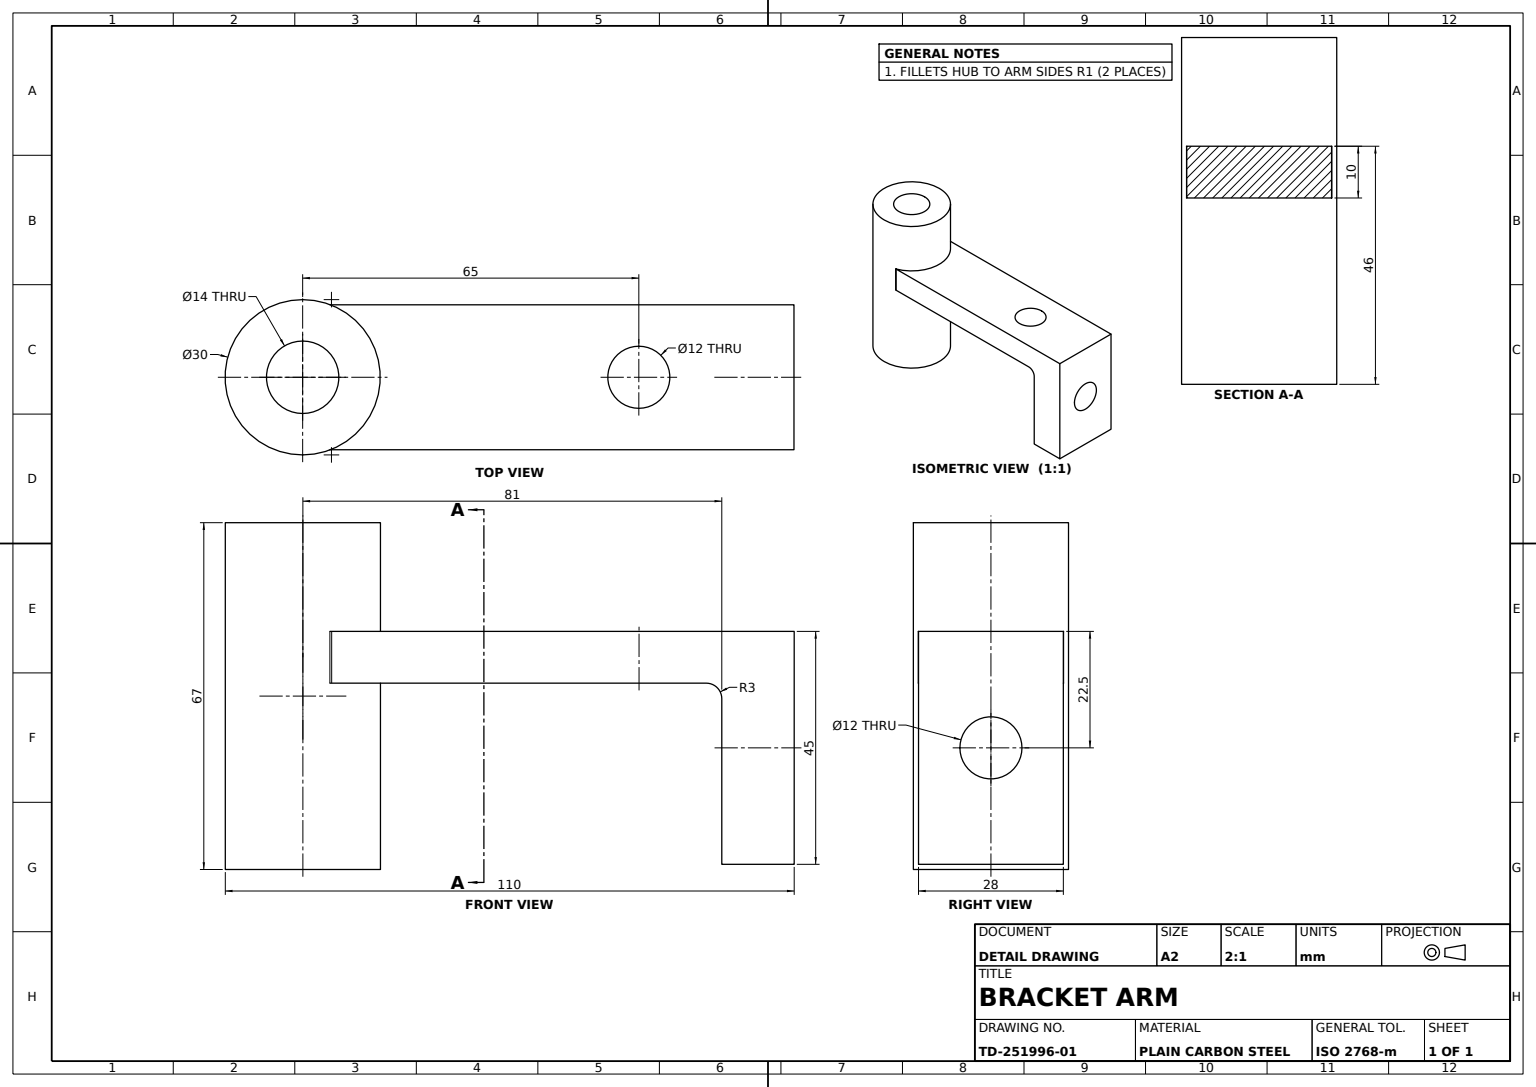
from build123d import *

# Parameters (mm, degrees)
CRANK_ARM_DEPTH        = 28
PIVOT_HUB_DEPTH        = 21
PIVOT_HUB_DEPTH_BACK   = 46
PIVOT_HUB_SKETCH_R     = 15
PIVOT_HUB_SKETCH_R_2   = 7
HUB_FILLET_R1_R        = 1
TOP_START              = 132
TOP_THROUGH_HOLE_DEPTH = 132
ARM_HOLE_SKETCH_R      = 6
ARM_THROUGH_HOLE_DEPTH = 132
BORE_SKETCH_R          = 6
THROUGH_BORE_DEPTH     = 42


with BuildPart() as part:
    # Arm Profile Sketch → Crank Arm (new body)
    with BuildSketch(Plane.XY):
        with BuildLine():
            Line((0, 0), (78, 0))
            ThreePointArc((78, 0), (80.121320344, -0.878679656), (81, -3))
            Line((81, -3), (81, -35))
            Line((81, -35), (95, -35))
            Line((95, -35), (95, 10))
            Line((95, 10), (0, 10))
            Line((0, 10), (0, 0))
        make_face()
    extrude(amount=CRANK_ARM_DEPTH)

    # Pivot Hub Sketch → Pivot Hub (add, two sides: drawn at the far end of the back side and taken through both)
    with BuildSketch(Plane(origin=(0, 10, 0), x_dir=(1, 0, 0), z_dir=(0, 1, 0)).offset(-PIVOT_HUB_DEPTH_BACK)):
        with Locations(Location((0, -14, 0), (0, 0, 270))):
            Circle(PIVOT_HUB_SKETCH_R)
        with Locations(Location((0, -14, 0), (0, 0, 270))):
            Circle(PIVOT_HUB_SKETCH_R_2, mode=Mode.SUBTRACT)
    extrude(amount=PIVOT_HUB_DEPTH + PIVOT_HUB_DEPTH_BACK)

    # Hub Fillet R1
    hub_fillet_r1_edges = [part.edges().sort_by_distance(p)[0] for p in [
        (5.385164807, 5, 0),
        (5.385164807, 5, 28),
    ]]
    fillet(hub_fillet_r1_edges, radius=HUB_FILLET_R1_R)

    # Top Hole Sketch → Top Through Hole (cut)
    with BuildSketch(Plane(origin=(0, 0, 0), x_dir=(1, 0, 0), z_dir=(0, 1, 0)).offset(TOP_START)):
        with BuildLine():
            Line((0, -7), (0, -21))
            ThreePointArc((0, -21), (7, -14), (0, -7))
        make_face()
    extrude(amount=-TOP_THROUGH_HOLE_DEPTH, mode=Mode.SUBTRACT)

    # Arm Hole Sketch → Arm Through Hole (cut)
    with BuildSketch(Plane(origin=(0, 10, 0), x_dir=(1, 0, 0), z_dir=(0, 1, 0))):
        with Locations(Location((65, -14, 0), (0, 0, 270))):
            Circle(ARM_HOLE_SKETCH_R)
    extrude(amount=-ARM_THROUGH_HOLE_DEPTH, mode=Mode.SUBTRACT)

    # Bore Sketch → Through Bore (cut)
    with BuildSketch(Plane(origin=(95, 0, 0), x_dir=(0, 0, -1), z_dir=(1, 0, 0))):
        with Locations((-14, -12.5)):
            Circle(BORE_SKETCH_R)
    extrude(amount=-THROUGH_BORE_DEPTH, mode=Mode.SUBTRACT)


solid = part.part
